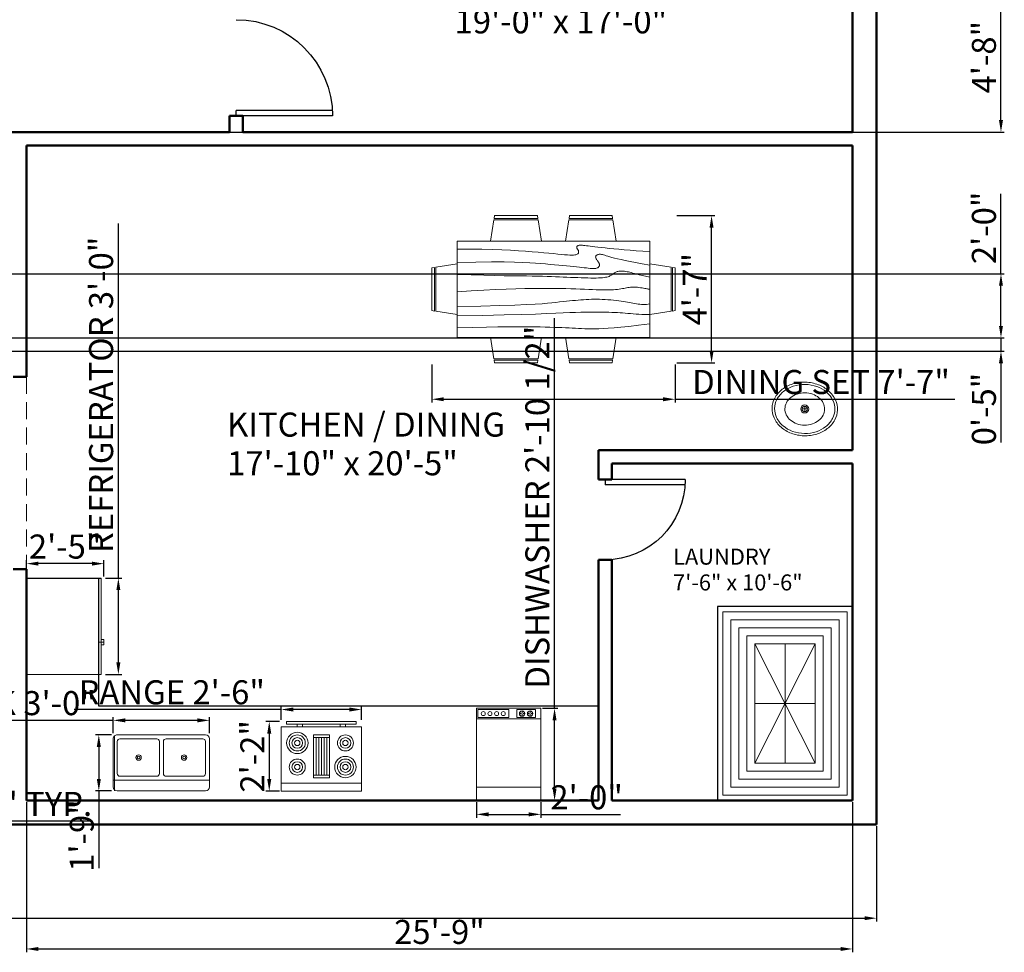
# Model space of a CAD drawing. Units: inches. Extents: x 2043 to 3102, y 1334 to 2053.
# Tile 3 of 4: x 2734 to 3102, y 1334 to 1683. Entities that reach past the tile are written whole.
import ezdxf

# ---------------------------------------------------------------- set-up
doc = ezdxf.new("R2010")
doc.units = ezdxf.units.IN
doc.linetypes.add('HIDDEN', pattern=[9.525, 6.35, -3.175])
for name, color, linetype, lineweight in [('A-ANNO-DIMS', 2, 'Continuous', 18), ('A-AREA-IDEN', 165, 'Continuous', 25), ('A-DOOR', 4, 'Continuous', 25), ('A-EQPM', 8, 'Continuous', 20), ('A-FLOR-CASE', 18, 'Continuous', 25), ('A-FLOR-FIXT', 9, 'Continuous', 20), ('A-FURN', 8, 'Continuous', 18), ('A-WALL', 7, 'Continuous', 50), ('A-WALL-OVHD', 11, 'HIDDEN', 18)]:
    doc.layers.add(name, color=color, linetype=linetype, lineweight=lineweight)
doc.styles.get("Standard").update_dxf_attribs({"font": 'arial.ttf'})
doc.dimstyles.new('ISO-25', dxfattribs={"dimtxt": 9, "dimasz": 4.5, "dimexe": 1.25, "dimexo": 0.625, "dimtad": 1, "dimdec": 0, "dimlunit": 3, "dimtxsty": 'Standard', "dimcen": 2.5, "dimadec": 0, "dimazin": 0, "dimtfac": 1, "dimtdec": 0, "dimtmove": 0, "dimatfit": 3, "dimfxl": 1, "dimarcsym": 0})

# ---------------------------------------------------------------- blocks, each defined once
blk = doc.blocks.new('Dining Set - 36 x 72 in.')
for p, q in [((-22.2343, 26.00059), (-23.4847, 17.99762)), ((-22.2304, 26), (-5.7608, 26)), ((-22, 27.5), (-22.1562, 26.50042)), ((-5.8416, 26.5), (-22.1534, 26.5)), ((-22, 27.5), (-6, 27.5)), ((-5.8437, 26.49966), (-6, 27.5)), ((-4.5152, 17.99762), (-5.7655, 25.99926)), ((5.7657, 26.00059), (4.5153, 17.99762)), ((5.7696, 26), (22.2392, 26)), ((6, 27.5), (5.8438, 26.50042)), ((22.1584, 26.5), (5.8466, 26.5)), ((6, 27.5), (22, 27.5)), ((22.1563, 26.49966), (22, 27.5)), ((23.4848, 17.99762), (22.2345, 25.99926)), ((36, 18), (-36, 18)), ((-36, 18), (-36, -18)), ((36, -18), (36, 18)), ((-45.5, 8), (-44.5004, 8.15617)), ((-45.5, 8), (-45.5, -8)), ((-44.5, -8.15843), (-44.5, 8.15338)), ((-44.0006, 8.23428), (-35.9976, 9.48474)), ((-44, 8.23041), (-44, -8.23915)), ((44.0006, 8.23428), (35.9976, 9.48474)), ((44, 8.23041), (44, -8.23915)), ((44.5, -8.15843), (44.5, 8.15338)), ((45.5, 8), (44.5005, 8.15617)), ((45.5, 8), (45.5, -8)), ((-44.4997, -8.15631), (-45.5, -8)), ((-35.9976, -9.48476), (-43.9993, -8.2345)), ((35.9976, -9.48476), (43.9993, -8.2345)), ((44.4997, -8.15631), (45.5, -8)), ((-36, -18), (36, -18)), ((-22.2343, -26.0006), (-23.4847, -17.99762)), ((-4.5152, -17.99762), (-5.7655, -25.99928)), ((5.7657, -26.0006), (4.5153, -17.99762)), ((23.4848, -17.99762), (22.2345, -25.99928)), ((-22.2304, -26), (-5.7608, -26)), ((-22, -27.5), (-22.1562, -26.50044)), ((-5.8416, -26.5), (-22.1534, -26.5)), ((-22, -27.5), (-6, -27.5)), ((-5.8437, -26.49967), (-6, -27.5)), ((5.7696, -26), (22.2392, -26)), ((6, -27.5), (5.8438, -26.50044)), ((22.1584, -26.5), (5.8466, -26.5)), ((6, -27.5), (22, -27.5)), ((22.1563, -26.49967), (22, -27.5))]:
    blk.add_line(p, q)
for points in [[(-36, 15), (-31.1772, 14.97754), (-26.8079, 14.91406), (-22.8538, 14.81543), (-19.276, 14.6875), (-16.0362, 14.53613), (-13.0957, 14.36718), (-10.4159, 14.18652), (-7.9583, 14), (-5.6904, 13.81315), (-3.6035, 13.63021), (-1.6954, 13.45508), (0.0365, 13.29166), (1.5945, 13.14388), (2.9811, 13.01562), (4.1988, 12.9108), (5.25, 12.83333), (6.1393, 12.78613), (6.8802, 12.76823), (7.4883, 12.77767), (7.9792, 12.8125), (8.3685, 12.87077), (8.6719, 12.95052), (8.9049, 13.0498), (9.0833, 13.16666), (9.2205, 13.29899), (9.3216, 13.44401), (9.3895, 13.59879), (9.4271, 13.76041), (9.4373, 13.92594), (9.4232, 14.09245), (9.3875, 14.257), (9.3333, 14.41666), (9.2638, 14.56917), (9.1836, 14.71484), (9.0975, 14.85465), (9.0104, 14.98958), (8.9272, 15.1206), (8.8529, 15.2487), (8.7922, 15.37483), (8.75, 15.5), (8.7305, 15.62467), (8.7344, 15.74739), (8.7617, 15.86621), (8.8125, 15.97916), (8.8867, 16.08431), (8.9844, 16.17968), (9.1055, 16.26334), (9.25, 16.33333), (9.4189, 16.38802), (9.6172, 16.42708), (9.8506, 16.45052), (10.125, 16.45833), (10.4463, 16.45052), (10.8203, 16.42708), (11.2529, 16.38802), (11.75, 16.33333), (12.3184, 16.26318), (12.9694, 16.17838), (13.7151, 16.07991), (14.5677, 15.96875), (15.5395, 15.84586), (16.6426, 15.71224), (17.8893, 15.56884), (19.2917, 15.41666), (20.859, 15.25667), (22.5879, 15.08984), (24.4721, 14.91715), (26.5052, 14.73958), (28.6809, 14.5581), (30.9929, 14.3737), (33.4347, 14.18733), (36, 14)], [(-36, 10), (-28.9766, 10.14274), (-23.1725, 10.20442), (-18.4241, 10.19775), (-14.5677, 10.13541), (-11.4399, 10.03011), (-8.877, 9.89453), (-6.7154, 9.74137), (-4.7917, 9.58333), (-2.9698, 9.43082), (-1.2246, 9.28515), (0.4415, 9.14534), (2.026, 9.01041), (3.5266, 8.87939), (4.9408, 8.7513), (6.266, 8.62516), (7.5, 8.5), (8.6411, 8.37549), (9.6914, 8.2539), (10.6538, 8.13818), (11.5312, 8.03125), (12.3267, 7.93603), (13.043, 7.85547), (13.6831, 7.79248), (14.25, 7.75), (14.7471, 7.7303), (15.1797, 7.73307), (15.5537, 7.75732), (15.875, 7.80208), (16.1494, 7.86637), (16.3828, 7.94922), (16.5811, 8.04964), (16.75, 8.16666), (16.8944, 8.29915), (17.0143, 8.44531), (17.1089, 8.60319), (17.1771, 8.77083), (17.218, 8.94629), (17.2305, 9.1276), (17.2137, 9.31282), (17.1667, 9.5), (17.0895, 9.6875), (16.987, 9.875), (16.8649, 10.0625), (16.7292, 10.25), (16.5856, 10.4375), (16.4401, 10.625), (16.2985, 10.8125), (16.1667, 11), (16.05, 11.18733), (15.9518, 11.3737), (15.8752, 11.5581), (15.8229, 11.73958), (15.798, 11.91715), (15.8034, 12.08984), (15.842, 12.25667), (15.9167, 12.41666), (16.0295, 12.56836), (16.1784, 12.70833), (16.3605, 12.83268), (16.5729, 12.9375), (16.8127, 13.01888), (17.0768, 13.07291), (17.3625, 13.0957), (17.6667, 13.08333), (17.9894, 13.03312), (18.3418, 12.94726), (18.7382, 12.82918), (19.1927, 12.68229), (19.7195, 12.51001), (20.3327, 12.31575), (21.0465, 12.10294), (21.875, 11.875), (22.8357, 11.63354), (23.959, 11.37304), (25.2786, 11.08618), (26.8282, 10.76562), (28.6414, 10.40405), (30.752, 9.99414), (33.1936, 9.52856), (36, 9)], [(-36, 5.5), (-30.7157, 5.3348), (-26.069, 5.20963), (-21.9946, 5.11767), (-18.4271, 5.05208), (-15.3009, 5.00602), (-12.5508, 4.97265), (-10.1112, 4.94515), (-7.9167, 4.91666), (-5.909, 4.88167), (-4.0586, 4.83984), (-2.3429, 4.79215), (-0.7396, 4.73958), (0.7739, 4.6831), (2.22, 4.6237), (3.6213, 4.56233), (5, 4.5), (6.373, 4.43782), (7.7344, 4.3776), (9.0723, 4.32129), (10.375, 4.27083), (11.6309, 4.22819), (12.8281, 4.19531), (13.9551, 4.17415), (15, 4.16666), (15.954, 4.17448), (16.819, 4.19791), (17.6001, 4.23698), (18.3021, 4.29166), (18.9299, 4.36198), (19.4883, 4.44791), (19.9823, 4.54948), (20.4167, 4.66666), (20.7969, 4.79899), (21.1302, 4.94401), (21.4245, 5.09879), (21.6875, 5.26041), (21.9271, 5.42594), (22.1511, 5.59245), (22.3672, 5.757), (22.5834, 5.91666), (22.8065, 6.06868), (23.0404, 6.21093), (23.2879, 6.34147), (23.5521, 6.45833), (23.8358, 6.55957), (24.142, 6.64323), (24.4735, 6.70735), (24.8334, 6.75), (25.2235, 6.76969), (25.642, 6.76692), (26.0858, 6.74267), (26.5521, 6.69791), (27.0379, 6.63362), (27.5404, 6.55078), (28.0565, 6.45036), (28.5834, 6.33333), (29.1242, 6.19987), (29.7071, 6.04687), (30.3661, 5.87044), (31.1354, 5.66666), (32.0493, 5.43164), (33.142, 5.16146), (34.4475, 4.85221), (36, 4.5)], [(-36, -1), (-30.7915, -0.6591), (-26.0195, -0.38216), (-21.6519, -0.16284), (-17.6563, 0.00521), (-14.0005, 0.12833), (-10.6523, 0.21289), (-7.5796, 0.26522), (-4.75, 0.29166), (-2.134, 0.29793), (0.2878, 0.28711), (2.5317, 0.26163), (4.6146, 0.22396), (6.5529, 0.17651), (8.3633, 0.12174), (10.0623, 0.06209), (11.6667, 0), (13.1899, -0.06201), (14.6341, -0.1211), (15.9982, -0.17432), (17.2813, -0.21875), (18.4823, -0.25147), (19.6003, -0.26953), (20.6343, -0.27002), (21.5834, -0.25), (22.4481, -0.20768), (23.2357, -0.14584), (23.9549, -0.06836), (24.6146, 0.02083), (25.2235, 0.11784), (25.7904, 0.21875), (26.3241, 0.31966), (26.8334, 0.41666), (27.3265, 0.50618), (27.8099, 0.58593), (28.2894, 0.65397), (28.7709, 0.70833), (29.2601, 0.74707), (29.763, 0.76823), (30.2855, 0.76985), (30.8334, 0.75), (31.4088, 0.70784), (31.9994, 0.64713), (32.589, 0.57275), (33.1615, 0.48958), (33.7008, 0.4025), (34.1908, 0.3164), (34.6153, 0.23616), (34.9584, 0.16666), (35.2099, 0.11165), (35.3848, 0.07031), (35.504, 0.04069), (35.5886, 0.02083), (35.6594, 0.00879), (35.7377, 0.0026), (35.8442, 0.00032), (36, 0)], [(-36, -6.5), (-27.1843, -6.31267), (-20.084, -6.1263), (-14.469, -5.9419), (-10.1094, -5.76042), (-6.7752, -5.58285), (-4.2363, -5.41016), (-2.2629, -5.24333), (-0.625, -5.08334), (0.8708, -4.93099), (2.2715, -4.78646), (3.5872, -4.64974), (4.8281, -4.52084), (6.0046, -4.39974), (7.127, -4.28646), (8.2053, -4.18099), (9.25, -4.08334), (10.2705, -3.99382), (11.2734, -3.91407), (12.2647, -3.84603), (13.25, -3.79167), (14.2354, -3.75293), (15.2266, -3.73177), (16.2295, -3.73015), (17.25, -3.75), (18.2912, -3.79248), (19.3451, -3.85547), (20.4009, -3.93604), (21.4479, -4.03125), (22.4754, -4.13819), (23.4727, -4.25391), (24.4289, -4.37549), (25.3334, -4.5), (26.1785, -4.62492), (26.9694, -4.74935), (27.7145, -4.87281), (28.4219, -4.99479), (29.1, -5.11483), (29.7572, -5.23242), (30.4016, -5.34709), (31.0417, -5.45834), (31.6837, -5.56437), (32.3262, -5.65821), (32.9658, -5.73153), (33.599, -5.77604), (34.2224, -5.78345), (34.8327, -5.74545), (35.4264, -5.65373), (36, -5.5)], [(-36, -10), (-26.4022, -9.81299), (-18.4675, -9.62891), (-11.9839, -9.45069), (-6.7396, -9.28125), (-2.5226, -9.12354), (0.8789, -8.98047), (3.6769, -8.85498), (6.0833, -8.75), (8.2767, -8.66765), (10.3021, -8.60677), (12.1712, -8.56543), (13.8958, -8.54167), (15.4876, -8.53353), (16.9583, -8.53907), (18.3197, -8.55632), (19.5834, -8.58334), (20.7616, -8.61841), (21.8685, -8.66081), (22.9188, -8.71004), (23.9271, -8.76563), (24.9081, -8.82707), (25.8763, -8.89388), (26.8465, -8.96558), (27.8334, -9.04167), (28.8474, -9.12118), (29.8828, -9.20117), (30.93, -9.27824), (31.9792, -9.34896), (33.0205, -9.40991), (34.0443, -9.45768), (35.0407, -9.48885), (36, -9.5)], [(-36, -14.5), (-30.0881, -14.33513), (-25.0332, -14.21224), (-20.7312, -14.12647), (-17.0781, -14.07292), (-13.97, -14.04671), (-11.3027, -14.04297), (-8.9724, -14.05681), (-6.875, -14.08334), (-4.9224, -14.11833), (-3.0905, -14.16016), (-1.3709, -14.20785), (0.2448, -14.26042), (1.7647, -14.3169), (3.1973, -14.3763), (4.5507, -14.43767), (5.8333, -14.5), (7.0554, -14.5621), (8.235, -14.62175), (9.3922, -14.67652), (10.5469, -14.72396), (11.7192, -14.76164), (12.929, -14.78711), (14.1965, -14.79794), (15.5417, -14.79167), (16.9933, -14.76424), (18.6152, -14.70508), (20.4804, -14.60197), (22.6615, -14.44271), (25.2312, -14.21509), (28.2624, -13.9069), (31.8277, -13.50594), (36, -13)]]:
    blk.add_lwpolyline(points)
blk = doc.blocks.new('Sink - Oval top')
for p, q in [((-1, 0), (1, 0)), ((0, 1), (0, -1))]:
    blk.add_line(p, q)
for points in [[(-12.23, 0.39, 0.117634), (-11.46, -3.36, 0.104469), (-8.88, -6.8, 0.090016), (-5.08, -9.07, 0.08192), (-0.32, -10.02, 0.08192), (4.49, -9.38, 0.090016), (8.42, -7.36, 0.104469), (11.22, -4.09, 0.117634), (12.23, -0.39, 0.117634), (11.46, 3.36, 0.104469), (8.88, 6.8, 0.090016), (5.08, 9.07, 0.08192), (0.32, 10.02, 0.08192), (-4.49, 9.38, 0.090016), (-8.42, 7.36, 0.104469), (-11.22, 4.09, 0.117634)], [(-11.29, 0.16, 0.118622), (-10.52, -3.25, 0.104678), (-8.07, -6.36, 0.089562), (-4.54, -8.37, 0.081185), (-0.13, -9.15, 0.081185), (4.3, -8.49, 0.089562), (7.89, -6.58, 0.104678), (10.42, -3.55, 0.118622), (11.29, -0.16, 0.118622), (10.52, 3.25, 0.104678), (8.07, 6.36, 0.089562), (4.54, 8.37, 0.081185), (0.13, 9.15, 0.081185), (-4.3, 8.49, 0.089562), (-7.89, 6.58, 0.104678), (-10.42, 3.55, 0.118622)], [(-7.42, 0.08, 0.118283), (-6.91, -2.17, 0.104607), (-5.29, -4.21, 0.089718), (-2.97, -5.53, 0.081436), (-0.07, -6.04, 0.081436), (2.84, -5.59, 0.089718), (5.2, -4.33, 0.104607), (6.86, -2.32, 0.118283), (7.42, -0.08, 0.118283), (6.91, 2.17, 0.104607), (5.29, 4.21, 0.089718), (2.97, 5.53, 0.081436), (0.07, 6.04, 0.081436), (-2.84, 5.59, 0.089718), (-5.2, 4.33, 0.104607), (-6.86, 2.32, 0.118283)]]:
    blk.add_lwpolyline(points, format="xyb", close=True)
for radius in [1.5, 1]:
    blk.add_circle((0, 0), radius)
blk = doc.blocks.new('Refrigerator-2 door - 36 in top')
for p, q in [((0, -26.999999), (36, -26.999999)), ((11, -27.999999), (11, -28.999999)), ((11, -28.999999), (13, -28.999999)), ((12, -26.999999), (12, -28.999999)), ((13, -28.999999), (13, -27.999999))]:
    blk.add_line(p, q)
blk.add_lwpolyline([(0, -27.999999), (0, 0), (36, 0), (36, -27.999999)], close=True)
blk = doc.blocks.new('Range-Oven - 30 in top')
for p, q in [((0, -3), (30, -3)), ((12, -6), (18, -6)), ((13, -20), (13, -6)), ((14, -6), (14, -20)), ((15, -20), (15, -6)), ((16, -6), (16, -20)), ((17, -20), (17, -6)), ((18, -20), (12, -20)), ((6, -24), (6, -25)), ((8, -25), (8, -24)), ((22, -25), (22, -24)), ((24, -24), (24, -25))]:
    blk.add_line(p, q)
for points in [[(0, -24), (0, 0), (30, 0), (30, -24)], [(12, -21), (12, -5), (18, -5), (18, -21)], [(2, -26), (2, -25), (28, -25), (28, -26)]]:
    blk.add_lwpolyline(points, close=True)
for centre, radius in [((6, -9), 4), ((6, -9), 3), ((6, -9), 2), ((24, -9), 3), ((24, -9), 2), ((6, -9), 1), ((24, -9), 1), ((24, -18), 4), ((6, -18), 3), ((6, -18), 2), ((6, -18), 1), ((24, -18), 3), ((24, -18), 2), ((24, -18), 1)]:
    blk.add_circle(centre, radius)
blk = doc.blocks.new('Dishwasher')
for p, q in [((16.3156, 33.1843), (16.5, 33)), ((17, 32.75), (17, 33.5)), ((17.5, 33), (17.6938, 33.1938)), ((19.3156, 33.1843), (19.5, 33)), ((20, 32.75), (20, 33.5)), ((20.5, 33), (20.6938, 33.1938)), ((24, 30.5), (0, 30.5)), ((16, 32.5), (16.75, 32.5)), ((16.5, 32), (16.2942, 31.7942)), ((17, 32.25), (17, 31.5)), ((18, 32.5), (17.25, 32.5)), ((17.7061, 31.7939), (17.5, 32)), ((19, 32.5), (19.75, 32.5)), ((19.5, 32), (19.2942, 31.7942)), ((20, 32.25), (20, 31.5)), ((21, 32.5), (20.25, 32.5)), ((20.7061, 31.7939), (20.5, 32)), ((0, 5), (24, 5))]:
    blk.add_line(p, q)
for points in [[(0, 0), (0, 34.5), (24, 34.5), (24, 0)], [(0.5, 31), (0.5, 34), (12, 34), (12, 31)], [(15, 31), (15, 34), (22, 34), (22, 31)]]:
    blk.add_lwpolyline(points, close=True)
for centre, radius in [((2.5, 32.5), 0.75), ((5, 32.5), 0.75), ((7.5, 32.5), 0.75), ((10, 32.5), 0.75), ((17, 32.5), 1), ((20, 32.5), 1)]:
    blk.add_circle(centre, radius)
blk = doc.blocks.new('Sink-double - 36 in top')
for p, q in [((-18, -4), (18, -4)), ((-0.75, -18.5), (-0.75, -6.5)), ((0.75, -6.5), (0.75, -18.5))]:
    blk.add_line(p, q)
for points in [[(-16.5, 0), (16.5, 0)], [(-18, -19.5), (-18, -1.5)], [(18, -1.5), (18, -19.5)], [(-16.5, -18.5), (-16.5, -6.5)], [(-15.5, -5.5), (-1.75, -5.5)], [(1.75, -5.5), (15.5, -5.5)], [(16.5, -6.5), (16.5, -18.5)], [(16.5, -21), (-16.5, -21)], [(-1.75, -19.5), (-15.5, -19.5)], [(15.5, -19.5), (1.75, -19.5)]]:
    blk.add_lwpolyline(points)
for centre, radius in [((-8.5, -12.5), 1), ((-8.5, -12.5), 0.5), ((8.5, -12.5), 1), ((8.5, -12.5), 0.5)]:
    blk.add_circle(centre, radius)
for centre, radius, start, end in [((-16.5, -1.5), 1.5, 90, 180), ((16.5, -1.5), 1.5, 0, 90), ((-15.5, -6.5), 1, 90, 180), ((-1.75, -6.5), 1, 0, 90), ((1.75, -6.5), 1, 90, 180), ((15.5, -6.5), 1, 0, 90), ((-16.5, -19.5), 1.5, 180, 270), ((-15.5, -18.5), 1, 180, 270), ((-1.75, -18.5), 1, 270, 0), ((1.75, -18.5), 1, 180, 270), ((15.5, -18.5), 1, 270, 0), ((16.5, -19.5), 1.5, 270, 0)]:
    blk.add_arc(centre, radius, start, end)
blk = doc.blocks.new('*D20')
at = {"layer": 'A-ANNO-DIMS', "color": 0, "lineweight": -2, "transparency": 16777216}
for p, q in [((2175.19, 1381.63), (2175.19, 1346)), ((3054.19, 1381.63), (3054.19, 1346)), ((2179.69, 1347.25), (3049.69, 1347.25))]:
    blk.add_line(p, q, dxfattribs=at)
at = {"layer": 'A-ANNO-DIMS', "color": 0, "transparency": 16777216}
for points in [[(2179.69, 1348), (2179.69, 1346.5), (2175.19, 1347.25)], [(3049.69, 1348), (3049.69, 1346.5), (3054.19, 1347.25)]]:
    blk.add_solid(points, dxfattribs=at)
at = {"layer": 'Defpoints', "color": 0, "transparency": 16777216}
for p in [(2175.19, 1382.25), (3054.19, 1382.25), (3054.19, 1347.25)]:
    blk.add_point(p, dxfattribs=at)
at = {"layer": 'A-ANNO-DIMS', "color": 0, "transparency": 16777216, "insert": (2614.69, 1352.47), "char_height": 9, "attachment_point": 5}
blk.add_mtext('73\'-3"', dxfattribs=at)
blk = doc.blocks.new('DOOR-SWING-30IN')
for p, q in [((0, 30), (30, 30)), ((30, 30), (30, 28)), ((0, 28), (30, 28))]:
    blk.add_line(p, q)
blk.add_arc((30, 30), 30, 180, 270)
blk = doc.blocks.new('DOOR-SWING-36IN')
for p, q in [((0, 36), (0, 0)), ((2, 36), (2, 0)), ((0, 0), (2, 0))]:
    blk.add_line(p, q)
blk.add_arc((0, 0), 36, 0, 90)
blk = doc.blocks.new('*D39')
at = {"layer": 'A-ANNO-DIMS', "color": 0, "lineweight": -2, "transparency": 16777216}
for p, q in [((2680.19, 1386.13), (2680.19, 1382.35)), ((2701.19, 1386.13), (2701.19, 1382.35)), ((2684.69, 1383.6), (2696.69, 1383.6)), ((2701.19, 1383.6), (2760.95, 1383.6))]:
    blk.add_line(p, q, dxfattribs=at)
at = {"layer": 'A-ANNO-DIMS', "color": 0, "transparency": 16777216}
for points in [[(2684.69, 1384.35), (2684.69, 1382.85), (2680.19, 1383.6)], [(2696.69, 1384.35), (2696.69, 1382.85), (2701.19, 1383.6)]]:
    blk.add_solid(points, dxfattribs=at)
at = {"layer": 'Defpoints', "color": 0, "transparency": 16777216}
for p in [(2680.19, 1386.75), (2701.19, 1386.75), (2701.19, 1383.6)]:
    blk.add_point(p, dxfattribs=at)
at = {"layer": 'A-ANNO-DIMS', "color": 0, "transparency": 16777216, "insert": (2733.32, 1388.82), "char_height": 9, "attachment_point": 5}
blk.add_mtext('1\'-9" TYP.', dxfattribs=at)
blk = doc.blocks.new('*D44')
at = {"layer": 'A-ANNO-DIMS', "color": 0, "lineweight": -2, "transparency": 16777216}
for p, q in [((2887.81, 1554.34), (2887.81, 1540.07)), ((2978.81, 1554.34), (2978.81, 1540.07)), ((2892.31, 1541.32), (2974.31, 1541.32)), ((2978.81, 1541.32), (3083.48, 1541.32))]:
    blk.add_line(p, q, dxfattribs=at)
at = {"layer": 'A-ANNO-DIMS', "color": 0, "transparency": 16777216}
for points in [[(2892.31, 1542.07), (2892.31, 1540.57), (2887.81, 1541.32)], [(2974.31, 1542.07), (2974.31, 1540.57), (2978.81, 1541.32)]]:
    blk.add_solid(points, dxfattribs=at)
at = {"layer": 'Defpoints', "color": 0, "transparency": 16777216}
for p in [(2887.81, 1554.97), (2978.81, 1554.97), (2978.81, 1541.32)]:
    blk.add_point(p, dxfattribs=at)
at = {"layer": 'A-ANNO-DIMS', "color": 0, "transparency": 16777216, "insert": (3033.4, 1546.59), "char_height": 9, "attachment_point": 5}
blk.add_mtext('DINING SET 7\'-7"', dxfattribs=at)
blk = doc.blocks.new('*D45')
at = {"layer": 'A-ANNO-DIMS', "color": 0, "lineweight": -2, "transparency": 16777216}
for p, q in [((2979.44, 1609.97), (2993.71, 1609.97)), ((2992.46, 1559.47), (2992.46, 1605.47)), ((2979.44, 1554.97), (2993.71, 1554.97))]:
    blk.add_line(p, q, dxfattribs=at)
at = {"layer": 'A-ANNO-DIMS', "color": 0, "transparency": 16777216}
for points in [[(2991.71, 1605.47), (2993.21, 1605.47), (2992.46, 1609.97)], [(2991.71, 1559.47), (2993.21, 1559.47), (2992.46, 1554.97)]]:
    blk.add_solid(points, dxfattribs=at)
at = {"layer": 'Defpoints', "color": 0, "transparency": 16777216}
for p in [(2978.81, 1609.97), (2992.46, 1609.97), (2978.81, 1554.97)]:
    blk.add_point(p, dxfattribs=at)
at = {"layer": 'A-ANNO-DIMS', "color": 0, "transparency": 16777216, "insert": (2987.34, 1582.47), "char_height": 9, "attachment_point": 5, "rotation": 90}
blk.add_mtext('4\'-7"', dxfattribs=at)
blk = doc.blocks.new('*D52')
at = {"layer": 'A-ANNO-DIMS', "color": 0, "lineweight": -2, "transparency": 16777216}
for p, q in [((2770.59, 1474.44), (2770.59, 1607.03)), ((2765.81, 1474.44), (2771.84, 1474.44)), ((2770.59, 1442.94), (2770.59, 1469.94)), ((2765.81, 1438.44), (2771.84, 1438.44))]:
    blk.add_line(p, q, dxfattribs=at)
at = {"layer": 'A-ANNO-DIMS', "color": 0, "transparency": 16777216}
for points in [[(2769.84, 1469.94), (2771.34, 1469.94), (2770.59, 1474.44)], [(2769.84, 1442.94), (2771.34, 1442.94), (2770.59, 1438.44)]]:
    blk.add_solid(points, dxfattribs=at)
at = {"layer": 'Defpoints', "color": 0, "transparency": 16777216}
for p in [(2765.19, 1474.44), (2770.59, 1474.44), (2765.19, 1438.44)]:
    blk.add_point(p, dxfattribs=at)
at = {"layer": 'A-ANNO-DIMS', "color": 0, "transparency": 16777216, "insert": (2765.3, 1542.98), "char_height": 9, "attachment_point": 5, "rotation": 90}
blk.add_mtext('REFRIGERATOR 3\'-0"', dxfattribs=at)
blk = doc.blocks.new('*D53')
at = {"layer": 'A-ANNO-DIMS', "color": 0, "lineweight": -2, "transparency": 16777216}
for p, q in [((2736.19, 1475.06), (2736.19, 1481.09)), ((2765.19, 1475.06), (2765.19, 1481.09)), ((2760.69, 1479.84), (2740.69, 1479.84))]:
    blk.add_line(p, q, dxfattribs=at)
at = {"layer": 'A-ANNO-DIMS', "color": 0, "transparency": 16777216}
for points in [[(2740.69, 1480.59), (2740.69, 1479.09), (2736.19, 1479.84)], [(2760.69, 1480.59), (2760.69, 1479.09), (2765.19, 1479.84)]]:
    blk.add_solid(points, dxfattribs=at)
at = {"layer": 'Defpoints', "color": 0, "transparency": 16777216}
for p in [(2736.19, 1479.84), (2736.19, 1474.44), (2765.19, 1474.44)]:
    blk.add_point(p, dxfattribs=at)
at = {"layer": 'A-ANNO-DIMS', "color": 0, "transparency": 16777216, "insert": (2750.69, 1485.06), "char_height": 9, "attachment_point": 5}
blk.add_mtext('2\'-5"', dxfattribs=at)
blk = doc.blocks.new('*D54')
at = {"layer": 'A-ANNO-DIMS', "color": 0, "lineweight": -2, "transparency": 16777216}
for p, q in [((2831.52, 1425.28), (2754.11, 1425.28)), ((2831.52, 1421.41), (2831.52, 1426.53)), ((2857.02, 1425.28), (2836.02, 1425.28)), ((2861.52, 1421.41), (2861.52, 1426.53))]:
    blk.add_line(p, q, dxfattribs=at)
at = {"layer": 'A-ANNO-DIMS', "color": 0, "transparency": 16777216}
for points in [[(2836.02, 1426.03), (2836.02, 1424.53), (2831.52, 1425.28)], [(2857.02, 1426.03), (2857.02, 1424.53), (2861.52, 1425.28)]]:
    blk.add_solid(points, dxfattribs=at)
at = {"layer": 'Defpoints', "color": 0, "transparency": 16777216}
for p in [(2831.52, 1425.28), (2831.52, 1420.78), (2861.52, 1420.78)]:
    blk.add_point(p, dxfattribs=at)
at = {"layer": 'A-ANNO-DIMS', "color": 0, "transparency": 16777216, "insert": (2790.56, 1430.56), "char_height": 9, "attachment_point": 5}
blk.add_mtext('RANGE 2\'-6"', dxfattribs=at)
blk = doc.blocks.new('*D55')
at = {"layer": 'A-ANNO-DIMS', "color": 0, "lineweight": -2, "transparency": 16777216}
for p, q in [((2830.89, 1420.78), (2825.77, 1420.78)), ((2827.02, 1416.28), (2827.02, 1399.28)), ((2830.89, 1394.78), (2825.77, 1394.78))]:
    blk.add_line(p, q, dxfattribs=at)
at = {"layer": 'A-ANNO-DIMS', "color": 0, "transparency": 16777216}
for points in [[(2826.27, 1416.28), (2827.77, 1416.28), (2827.02, 1420.78)], [(2826.27, 1399.28), (2827.77, 1399.28), (2827.02, 1394.78)]]:
    blk.add_solid(points, dxfattribs=at)
at = {"layer": 'Defpoints', "color": 0, "transparency": 16777216}
for p in [(2831.52, 1420.78), (2827.02, 1394.78), (2831.52, 1394.78)]:
    blk.add_point(p, dxfattribs=at)
at = {"layer": 'A-ANNO-DIMS', "color": 0, "transparency": 16777216, "insert": (2821.87, 1407.78), "char_height": 9, "attachment_point": 5, "rotation": 90}
blk.add_mtext('2\'-2"', dxfattribs=at)
blk = doc.blocks.new('*D56')
at = {"layer": 'A-ANNO-DIMS', "color": 0, "lineweight": -2, "transparency": 16777216}
for p, q in [((2933.74, 1425.75), (2933.74, 1571.66)), ((2929.19, 1425.75), (2934.99, 1425.75)), ((2933.74, 1395.75), (2933.74, 1421.25)), ((2929.19, 1391.25), (2934.99, 1391.25))]:
    blk.add_line(p, q, dxfattribs=at)
at = {"layer": 'A-ANNO-DIMS', "color": 0, "transparency": 16777216}
for points in [[(2932.99, 1421.25), (2934.49, 1421.25), (2933.74, 1425.75)], [(2932.99, 1395.75), (2934.49, 1395.75), (2933.74, 1391.25)]]:
    blk.add_solid(points, dxfattribs=at)
at = {"layer": 'Defpoints', "color": 0, "transparency": 16777216}
for p in [(2928.57, 1425.75), (2933.74, 1425.75), (2928.57, 1391.25)]:
    blk.add_point(p, dxfattribs=at)
at = {"layer": 'A-ANNO-DIMS', "color": 0, "transparency": 16777216, "insert": (2928.46, 1500.96), "char_height": 9, "attachment_point": 5, "rotation": 90}
blk.add_mtext('DISHWASHER 2\'-10 1/2"', dxfattribs=at)
blk = doc.blocks.new('*D57')
at = {"layer": 'A-ANNO-DIMS', "color": 0, "lineweight": -2, "transparency": 16777216}
for p, q in [((2904.57, 1390.63), (2904.57, 1384.83)), ((2928.57, 1390.63), (2928.57, 1384.83)), ((2909.07, 1386.08), (2924.07, 1386.08)), ((2928.57, 1386.08), (2958.39, 1386.08))]:
    blk.add_line(p, q, dxfattribs=at)
at = {"layer": 'A-ANNO-DIMS', "color": 0, "transparency": 16777216}
for points in [[(2909.07, 1386.83), (2909.07, 1385.33), (2904.57, 1386.08)], [(2924.07, 1386.83), (2924.07, 1385.33), (2928.57, 1386.08)]]:
    blk.add_solid(points, dxfattribs=at)
at = {"layer": 'Defpoints', "color": 0, "transparency": 16777216}
for p in [(2904.57, 1391.25), (2928.57, 1391.25), (2928.57, 1386.08)]:
    blk.add_point(p, dxfattribs=at)
at = {"layer": 'A-ANNO-DIMS', "color": 0, "transparency": 16777216, "insert": (2945.73, 1391.3), "char_height": 9, "attachment_point": 5}
blk.add_mtext('2\'-0"', dxfattribs=at)
blk = doc.blocks.new('*D58')
at = {"layer": 'A-ANNO-DIMS', "color": 0, "lineweight": -2, "transparency": 16777216}
for p, q in [((2768.68, 1416.46), (2768.68, 1422.48)), ((2804.68, 1416.46), (2804.68, 1422.48)), ((2768.68, 1421.23), (2651.42, 1421.23)), ((2800.18, 1421.23), (2773.18, 1421.23))]:
    blk.add_line(p, q, dxfattribs=at)
at = {"layer": 'A-ANNO-DIMS', "color": 0, "transparency": 16777216}
for points in [[(2773.18, 1421.98), (2773.18, 1420.48), (2768.68, 1421.23)], [(2800.18, 1421.98), (2800.18, 1420.48), (2804.68, 1421.23)]]:
    blk.add_solid(points, dxfattribs=at)
at = {"layer": 'Defpoints', "color": 0, "transparency": 16777216}
for p in [(2768.68, 1421.23), (2768.68, 1415.83), (2804.68, 1415.83)]:
    blk.add_point(p, dxfattribs=at)
at = {"layer": 'A-ANNO-DIMS', "color": 0, "transparency": 16777216, "insert": (2707.8, 1426.51), "char_height": 9, "attachment_point": 5}
blk.add_mtext('DOUBLE SINK 3\'-0"', dxfattribs=at)
blk = doc.blocks.new('*D59')
at = {"layer": 'A-ANNO-DIMS', "color": 0, "lineweight": -2, "transparency": 16777216}
for p, q in [((2768.06, 1415.83), (2762.03, 1415.83)), ((2763.28, 1411.33), (2763.28, 1399.33)), ((2768.06, 1394.83), (2762.03, 1394.83)), ((2763.28, 1394.83), (2763.28, 1366))]:
    blk.add_line(p, q, dxfattribs=at)
at = {"layer": 'A-ANNO-DIMS', "color": 0, "transparency": 16777216}
for points in [[(2762.53, 1411.33), (2764.03, 1411.33), (2763.28, 1415.83)], [(2762.53, 1399.33), (2764.03, 1399.33), (2763.28, 1394.83)]]:
    blk.add_solid(points, dxfattribs=at)
at = {"layer": 'Defpoints', "color": 0, "transparency": 16777216}
for p in [(2768.68, 1415.83), (2763.28, 1394.83), (2768.68, 1394.83)]:
    blk.add_point(p, dxfattribs=at)
at = {"layer": 'A-ANNO-DIMS', "color": 0, "transparency": 16777216, "insert": (2758.06, 1378.17), "char_height": 9, "attachment_point": 5, "rotation": 90}
blk.add_mtext('1\'-9"', dxfattribs=at)
blk = doc.blocks.new('*D60')
at = {"layer": 'A-ANNO-DIMS', "color": 0, "lineweight": -2, "transparency": 16777216}
for p, q in [((2423.81, 1697.25), (3101.95, 1697.25)), ((3100.7, 1645.75), (3100.7, 1692.75)), ((2417.81, 1641.25), (3101.95, 1641.25))]:
    blk.add_line(p, q, dxfattribs=at)
at = {"layer": 'A-ANNO-DIMS', "color": 0, "transparency": 16777216}
for points in [[(3099.95, 1692.75), (3101.45, 1692.75), (3100.7, 1697.25)], [(3099.95, 1645.75), (3101.45, 1645.75), (3100.7, 1641.25)]]:
    blk.add_solid(points, dxfattribs=at)
at = {"layer": 'Defpoints', "color": 0, "transparency": 16777216}
for p in [(2423.19, 1697.25), (3100.7, 1697.25), (2417.19, 1641.25)]:
    blk.add_point(p, dxfattribs=at)
at = {"layer": 'A-ANNO-DIMS', "color": 0, "transparency": 16777216, "insert": (3095.48, 1669.25), "char_height": 9, "attachment_point": 5, "rotation": 90}
blk.add_mtext('4\'-8"', dxfattribs=at)
blk = doc.blocks.new('*D62')
at = {"layer": 'A-ANNO-DIMS', "color": 0, "lineweight": -2, "transparency": 16777216}
for p, q in [((3100.7, 1588.25), (3100.7, 1618.08)), ((2352.81, 1588.25), (3101.95, 1588.25)), ((3100.7, 1568.75), (3100.7, 1583.75)), ((2352.81, 1564.25), (3101.95, 1564.25))]:
    blk.add_line(p, q, dxfattribs=at)
at = {"layer": 'A-ANNO-DIMS', "color": 0, "transparency": 16777216}
for points in [[(3099.95, 1583.75), (3101.45, 1583.75), (3100.7, 1588.25)], [(3099.95, 1568.75), (3101.45, 1568.75), (3100.7, 1564.25)]]:
    blk.add_solid(points, dxfattribs=at)
at = {"layer": 'Defpoints', "color": 0, "transparency": 16777216}
for p in [(2352.19, 1588.25), (3100.7, 1588.25), (2352.19, 1564.25)]:
    blk.add_point(p, dxfattribs=at)
at = {"layer": 'A-ANNO-DIMS', "color": 0, "transparency": 16777216, "insert": (3095.48, 1605.42), "char_height": 9, "attachment_point": 5, "rotation": 90}
blk.add_mtext('2\'-0"', dxfattribs=at)
blk = doc.blocks.new('*D64')
at = {"layer": 'A-ANNO-DIMS', "color": 0, "lineweight": -2, "transparency": 16777216}
for p, q in [((3100.7, 1568.75), (3100.7, 1573.25)), ((2352.81, 1564.25), (3101.95, 1564.25)), ((3100.7, 1564.25), (3100.7, 1559.25)), ((2352.81, 1559.25), (3101.95, 1559.25)), ((3100.7, 1554.75), (3100.7, 1525.08))]:
    blk.add_line(p, q, dxfattribs=at)
at = {"layer": 'A-ANNO-DIMS', "color": 0, "transparency": 16777216}
for points in [[(3099.95, 1568.75), (3101.45, 1568.75), (3100.7, 1564.25)], [(3099.95, 1554.75), (3101.45, 1554.75), (3100.7, 1559.25)]]:
    blk.add_solid(points, dxfattribs=at)
at = {"layer": 'Defpoints', "color": 0, "transparency": 16777216}
for p in [(2352.19, 1564.25), (2352.19, 1559.25), (3100.7, 1559.25)]:
    blk.add_point(p, dxfattribs=at)
at = {"layer": 'A-ANNO-DIMS', "color": 0, "transparency": 16777216, "insert": (3095.48, 1537.67), "char_height": 9, "attachment_point": 5, "rotation": 90}
blk.add_mtext('0\'-5"', dxfattribs=at)
blk = doc.blocks.new('*D65')
at = {"layer": 'A-ANNO-DIMS', "color": 0, "lineweight": -2, "transparency": 16777216}
for p, q in [((2736.19, 1390.63), (2736.19, 1334.49)), ((3045.19, 1390.63), (3045.19, 1334.49)), ((2740.69, 1335.74), (3040.69, 1335.74))]:
    blk.add_line(p, q, dxfattribs=at)
at = {"layer": 'A-ANNO-DIMS', "color": 0, "transparency": 16777216}
for points in [[(2740.69, 1336.49), (2740.69, 1334.99), (2736.19, 1335.74)], [(3040.69, 1336.49), (3040.69, 1334.99), (3045.19, 1335.74)]]:
    blk.add_solid(points, dxfattribs=at)
at = {"layer": 'Defpoints', "color": 0, "transparency": 16777216}
for p in [(2736.19, 1391.25), (3045.19, 1391.25), (3045.19, 1335.74)]:
    blk.add_point(p, dxfattribs=at)
at = {"layer": 'A-ANNO-DIMS', "color": 0, "transparency": 16777216, "insert": (2890.69, 1340.96), "char_height": 9, "attachment_point": 5}
blk.add_mtext('25\'-9"', dxfattribs=at)

msp = doc.modelspace()

# ---------------------------------------------------------------- linework, layer by layer
at = {"layer": 'A-EQPM'}
for p, q in [((3008.68, 1449.86), (3031.19, 1405.25)), ((3031.19, 1449.86), (3008.68, 1405.25)), ((3019.94, 1449.86), (3019.94, 1405.25)), ((3008.68, 1427.56), (3031.19, 1427.56))]:
    msp.add_line(p, q, dxfattribs=at)
for points in [[(3043.19, 1393.25), (3043.19, 1461.86), (2996.68, 1461.86), (2996.68, 1393.25)], [(3040.19, 1396.25), (3040.19, 1458.86), (2999.68, 1458.86), (2999.68, 1396.25)], [(3037.19, 1399.25), (3037.19, 1455.86), (3002.68, 1455.86), (3002.68, 1399.25)], [(3034.19, 1402.25), (3034.19, 1452.86), (3005.68, 1452.86), (3005.68, 1402.25)], [(3031.19, 1405.25), (3031.19, 1449.86), (3008.68, 1449.86), (3008.68, 1405.25)]]:
    msp.add_lwpolyline(points, close=True, dxfattribs=at)
at = {"layer": 'A-FLOR-CASE'}
for p, q in [((2736.19, 1474.44), (2764.19, 1474.44)), ((2763.19, 1474.44), (2763.19, 1426.72)), ((3045.19, 1463.86), (2994.68, 1463.86)), ((2994.68, 1463.86), (2994.68, 1391.25)), ((2763.19, 1426.72), (2950.19, 1426.72))]:
    msp.add_line(p, q, dxfattribs=at)
at = {"layer": 'A-FLOR-FIXT'}
msp.add_line((2769.12, 1394.83), (2769.12, 1415.39), dxfattribs=at)
at = {"layer": 'A-WALL'}
for p, q in [((3054.19, 1976.25), (3054.19, 1382.25)), ((3045.19, 1845.25), (3045.19, 1641.25)), ((2812.19, 1647.25), (2812.19, 1641.25)), ((2812.19, 1647.25), (2817.19, 1647.25)), ((2817.19, 1647.25), (2817.19, 1641.25)), ((2725.19, 1641.25), (2812.19, 1641.25)), ((2817.19, 1641.25), (3045.19, 1641.25)), ((2736.19, 1636.25), (2736.19, 1549.75)), ((2736.19, 1636.25), (3045.19, 1636.25)), ((3045.19, 1636.25), (3045.19, 1522.25)), ((2736.19, 1549.75), (2731.19, 1549.75)), ((2950.19, 1522.25), (3045.19, 1522.25)), ((2950.19, 1522.25), (2950.19, 1511.25)), ((2955.19, 1517.25), (3045.19, 1517.25)), ((2955.19, 1517.25), (2955.19, 1511.25)), ((3045.19, 1517.25), (3045.19, 1391.25)), ((2950.19, 1511.25), (2955.19, 1511.25)), ((2950.19, 1481.25), (2955.19, 1481.25)), ((2950.19, 1481.25), (2950.19, 1391.25)), ((2955.19, 1481.25), (2955.19, 1391.25)), ((2736.19, 1477.75), (2731.19, 1477.75)), ((2736.19, 1477.75), (2736.19, 1391.25)), ((2950.19, 1397.25), (2950.19, 1391.25)), ((2955.19, 1397.25), (2955.19, 1391.25)), ((2736.19, 1391.25), (2950.19, 1391.25)), ((2955.19, 1391.25), (3045.19, 1391.25)), ((2722.19, 1382.25), (3054.19, 1382.25))]:
    msp.add_line(p, q, dxfattribs=at)
at = {"layer": 'A-WALL-OVHD'}
msp.add_line((2736.19, 1549.75), (2736.19, 1474.44), dxfattribs=at)

# ---------------------------------------------------------------- block references
at = {"layer": 'A-DOOR', "extrusion": (0, 0, -1), "zscale": -1, "rotation": 90.0000000000006}
msp.add_blockref('DOOR-SWING-36IN', (-2814.69, 1647.26), dxfattribs=at)
at = {"layer": 'A-DOOR', "extrusion": (0, 0, -1), "zscale": -1}
msp.add_blockref('DOOR-SWING-30IN', (-2982.6, 1481.25), dxfattribs=at)
at = {"layer": 'A-EQPM'}
for name, p, rotation in [('Refrigerator-2 door - 36 in top', (2736.19, 1438.44), 90), ('Range-Oven - 30 in top', (2861.52, 1394.78), 180)]:
    msp.add_blockref(name, p, dxfattribs=dict(at, rotation=rotation))
msp.add_blockref('Dishwasher', (2904.57, 1391.25), dxfattribs=at)
at = {"layer": 'A-FLOR-FIXT'}
msp.add_blockref('Sink - Oval top', (3027.31, 1537.68), dxfattribs=at)
at = {"layer": 'A-FLOR-FIXT', "rotation": 180}
msp.add_blockref('Sink-double - 36 in top', (2786.68, 1394.83), dxfattribs=at)
at = {"layer": 'A-FURN'}
msp.add_blockref('Dining Set - 36 x 72 in.', (2933.31, 1582.47), dxfattribs=at)

# ---------------------------------------------------------------- texts
at = {"layer": 'A-AREA-IDEN'}
for s, height, p in [('19\'-0" x 17\'-0"', 9, (2896.35, 1678.13)), ('KITCHEN / DINING', 9, (2811.26, 1527.34)), ('17\'-10" x 20\'-5"', 9, (2811.26, 1512.88)), ('LAUNDRY', 6, (2978.05, 1479.45)), ('7\'-6" x 10\'-6"', 6, (2978.05, 1469.81))]:
    msp.add_text(s, height=height, dxfattribs=at).set_placement(p)

# ---------------------------------------------------------------- dimensions: what is measured, and where the dimension line sits
at = {"layer": 'A-ANNO-DIMS'}
for base, p1, p2, angle, picture, middle in [((3100.7, 1697.25), (2417.19, 1641.25), (2423.19, 1697.25), 90, '*D60', (3095.48, 1669.25)), ((3100.7, 1588.25), (2352.19, 1564.25), (2352.19, 1588.25), 90, '*D62', (3095.48, 1605.42)), ((2992.46, 1609.97), (2978.81, 1554.97), (2978.81, 1609.97), 90, '*D45', (2987.34, 1582.47)), ((3100.7, 1559.25), (2352.19, 1564.25), (2352.19, 1559.25), 90, '*D64', (3095.48, 1537.67)), ((2736.19, 1479.84), (2765.19, 1474.44), (2736.19, 1474.44), 180, '*D53', (2750.69, 1485.06)), ((2827.02, 1394.78), (2831.52, 1420.78), (2831.52, 1394.78), 270, '*D55', (2821.87, 1407.78)), ((2763.28, 1394.83), (2768.68, 1415.83), (2768.68, 1394.83), 270, '*D59', (2758.06, 1378.17))]:
    dim = msp.add_linear_dim(base=base, p1=p1, p2=p2, angle=angle, dimstyle='ISO-25', override={"dimdec": 1, "dimlfac": 1, "dimrnd": 0, "dimzin": 1, "dimdsep": 46, "dimlunit": 4, "dimfrac": 2}, dxfattribs=at)
    dim.commit()
    dim.dimension.update_dxf_attribs({"geometry": picture, "text_midpoint": middle})
for base, p1, p2, angle, text, picture, middle in [((2770.59, 1474.44), (2765.19, 1438.44), (2765.19, 1474.44), 90, 'REFRIGERATOR <>', '*D52', (2765.3, 1542.98)), ((2933.74, 1425.75), (2928.57, 1391.25), (2928.57, 1425.75), 90, 'DISHWASHER <>', '*D56', (2928.46, 1500.96)), ((2768.68, 1421.23), (2804.68, 1415.83), (2768.68, 1415.83), 180, 'DOUBLE SINK <>', '*D58', (2707.8, 1426.51)), ((2831.52, 1425.28), (2861.52, 1420.78), (2831.52, 1420.78), 180, 'RANGE <>', '*D54', (2790.56, 1430.56))]:
    dim = msp.add_linear_dim(base=base, p1=p1, p2=p2, angle=angle, text=text, dimstyle='ISO-25', override={"dimdec": 1, "dimlfac": 1, "dimrnd": 0, "dimzin": 1, "dimdsep": 46, "dimlunit": 4, "dimfrac": 2}, dxfattribs=at)
    dim.commit()
    dim.dimension.update_dxf_attribs({"geometry": picture, "text_midpoint": middle})
for base, p1, p2, text, picture, middle in [((2978.81, 1541.32), (2887.81, 1554.97), (2978.81, 1554.97), 'DINING SET <>', '*D44', (3033.4, 1546.59)), ((2701.19, 1383.6), (2680.19, 1386.75), (2701.19, 1386.75), '<> TYP.', '*D39', (2733.32, 1388.82))]:
    dim = msp.add_linear_dim(base=base, p1=p1, p2=p2, text=text, dimstyle='ISO-25', override={"dimdec": 1, "dimlfac": 1, "dimrnd": 0, "dimzin": 1, "dimdsep": 46, "dimlunit": 4, "dimfrac": 2}, dxfattribs=at)
    dim.commit()
    dim.dimension.update_dxf_attribs({"geometry": picture, "text_midpoint": middle})
for base, p1, p2, override, picture, middle in [((2928.57, 1386.08), (2904.57, 1391.25), (2928.57, 1391.25), {"dimdec": 1, "dimlfac": 1, "dimrnd": 0, "dimzin": 1, "dimdsep": 46, "dimlunit": 4, "dimfrac": 2}, '*D57', (2945.73, 1391.3)), ((3045.19, 1335.74), (2736.19, 1391.25), (3045.19, 1391.25), {"dimdec": 1, "dimlfac": 1, "dimrnd": 0, "dimzin": 1, "dimdsep": 46, "dimlunit": 4, "dimfrac": 2}, '*D65', (2890.69, 1340.96)), ((3054.19, 1347.25), (2175.19, 1382.25), (3054.19, 1382.25), {"dimclrd": 0, "dimclre": 0, "dimclrt": 0}, '*D20', (2614.69, 1352.47))]:
    dim = msp.add_linear_dim(base=base, p1=p1, p2=p2, dimstyle='ISO-25', override=override, dxfattribs=at)
    dim.commit()
    dim.dimension.update_dxf_attribs({"geometry": picture, "text_midpoint": middle})

doc.saveas('drawing.dxf')
